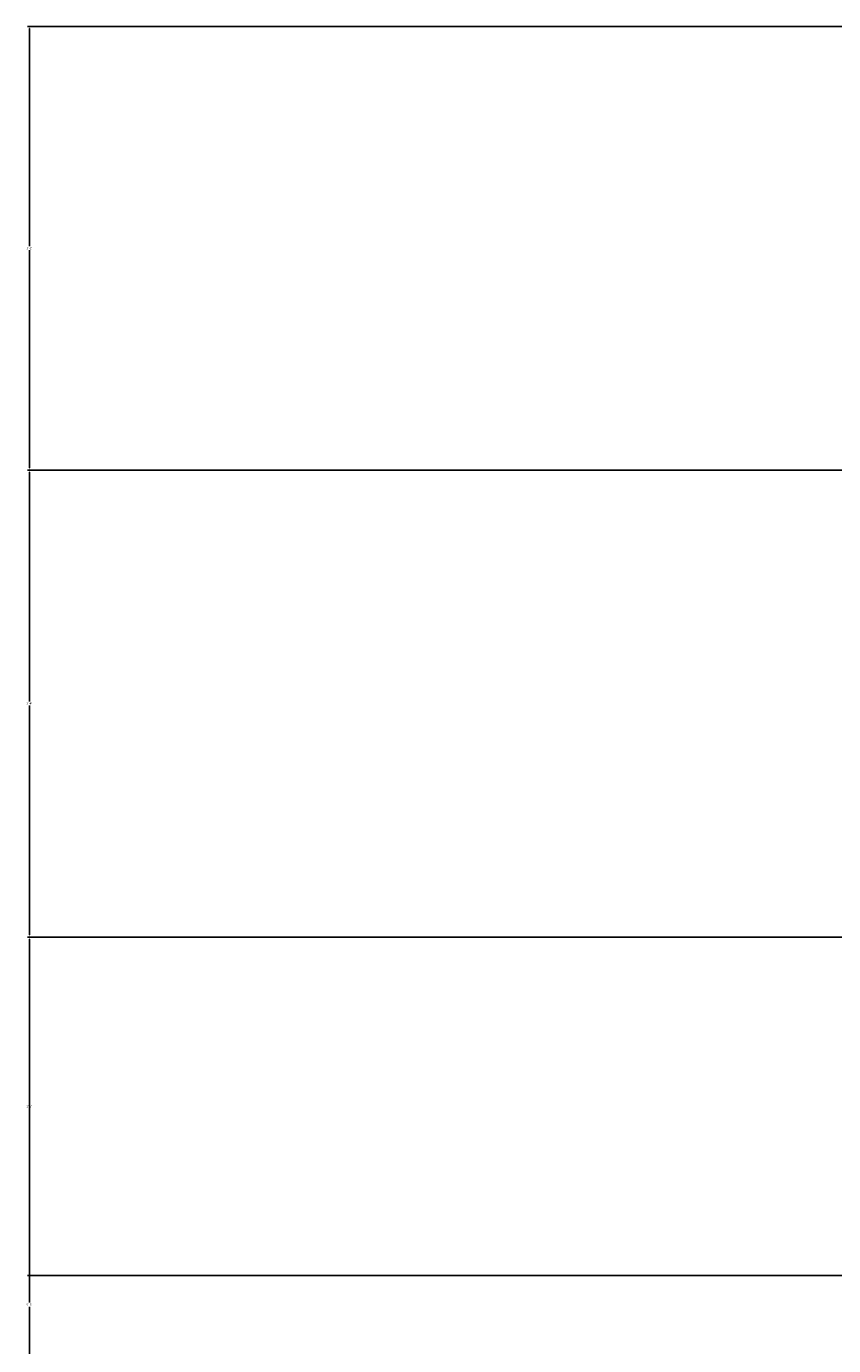
# Model space of a CAD drawing. Units: inches. Extents: x 37 to 824, y -700 to 234.
# Tile 49 of 77: x 78 to 147, y 78 to 191. Entities that reach past the tile are written whole.
import ezdxf

# ---------------------------------------------------------------- set-up
doc = ezdxf.new("R2010")
doc.units = ezdxf.units.IN
doc.header["$MEASUREMENT"] = 0
doc.layers.add('A-ANNO-DIMS', color=2, linetype='Continuous', lineweight=18)
doc.styles.get("Standard").update_dxf_attribs({"font": 'arial.ttf'})
doc.dimstyles.get("Standard").update_dxf_attribs({"dimtxt": 0.18, "dimasz": 0.18, "dimexe": 0.18, "dimexo": 0.0625, "dimgap": 0.09, "dimtad": 0, "dimtih": 1, "dimtoh": 1, "dimdec": 1, "dimzin": 0, "dimdsep": 46, "dimlunit": 4, "dimtxsty": 'Standard', "dimcen": 0.09, "dimadec": 0, "dimazin": 0, "dimtfac": 1, "dimtdec": 1, "dimtofl": 0, "dimtmove": 0, "dimatfit": 3, "dimfxl": 1, "dimtolj": 1, "dimtzin": 0, "dimarcsym": 0})

# ---------------------------------------------------------------- blocks, each defined once
blk = doc.blocks.new('*D49')
at = {"layer": 'A-ANNO-DIMS', "color": 0, "lineweight": -2, "ltscale": 0.5, "transparency": 16777216}
for p, q in [((161.01, 191.09), (78.16, 191.09)), ((78.34, 190.91), (78.34, 172.27)), ((78.34, 153.27), (78.34, 171.91)), ((161.01, 153.09), (78.16, 153.09))]:
    blk.add_line(p, q, dxfattribs=at)
at = {"layer": 'A-ANNO-DIMS', "color": 0, "ltscale": 0.5, "transparency": 16777216}
for points in [[(78.31, 190.91), (78.37, 190.91), (78.34, 191.09)], [(78.31, 153.27), (78.37, 153.27), (78.34, 153.09)]]:
    blk.add_solid(points, dxfattribs=at)
at = {"layer": 'Defpoints', "color": 0, "ltscale": 0.5, "transparency": 16777216}
for p in [(161.08, 191.09), (78.34, 153.09), (161.08, 153.09)]:
    blk.add_point(p, dxfattribs=at)
at = {"layer": 'A-ANNO-DIMS', "color": 0, "ltscale": 0.5, "transparency": 16777216, "insert": (78.34, 172.09), "char_height": 0.18, "attachment_point": 5}
blk.add_mtext('\\A1;3\'-2"', dxfattribs=at)
blk = doc.blocks.new('*D50')
at = {"layer": 'A-ANNO-DIMS', "color": 0, "lineweight": -2, "ltscale": 0.5, "transparency": 16777216}
for p, q in [((161.01, 153.09), (78.16, 153.09)), ((78.34, 152.91), (78.34, 133.27)), ((78.34, 113.27), (78.34, 132.91)), ((161.01, 113.09), (78.16, 113.09))]:
    blk.add_line(p, q, dxfattribs=at)
at = {"layer": 'A-ANNO-DIMS', "color": 0, "ltscale": 0.5, "transparency": 16777216}
for points in [[(78.31, 152.91), (78.37, 152.91), (78.34, 153.09)], [(78.31, 113.27), (78.37, 113.27), (78.34, 113.09)]]:
    blk.add_solid(points, dxfattribs=at)
at = {"layer": 'Defpoints', "color": 0, "ltscale": 0.5, "transparency": 16777216}
for p in [(161.08, 153.09), (78.34, 113.09), (161.08, 113.09)]:
    blk.add_point(p, dxfattribs=at)
at = {"layer": 'A-ANNO-DIMS', "color": 0, "ltscale": 0.5, "transparency": 16777216, "insert": (78.34, 133.09), "char_height": 0.18, "attachment_point": 5}
blk.add_mtext('\\A1;3\'-4"', dxfattribs=at)
blk = doc.blocks.new('*D51')
at = {"layer": 'A-ANNO-DIMS', "color": 0, "lineweight": -2, "ltscale": 0.5, "transparency": 16777216}
for p, q in [((161.01, 113.09), (78.16, 113.09)), ((78.34, 112.91), (78.34, 81.77)), ((78.34, 50.27), (78.34, 81.41)), ((161.01, 50.09), (78.16, 50.09))]:
    blk.add_line(p, q, dxfattribs=at)
at = {"layer": 'A-ANNO-DIMS', "color": 0, "ltscale": 0.5, "transparency": 16777216}
for points in [[(78.31, 112.91), (78.37, 112.91), (78.34, 113.09)], [(78.31, 50.27), (78.37, 50.27), (78.34, 50.09)]]:
    blk.add_solid(points, dxfattribs=at)
at = {"layer": 'Defpoints', "color": 0, "ltscale": 0.5, "transparency": 16777216}
for p in [(161.08, 113.09), (78.34, 50.09), (161.08, 50.09)]:
    blk.add_point(p, dxfattribs=at)
at = {"layer": 'A-ANNO-DIMS', "color": 0, "ltscale": 0.5, "transparency": 16777216, "insert": (78.34, 81.59), "char_height": 0.18, "attachment_point": 5}
blk.add_mtext('\\A1;5\'-3"', dxfattribs=at)
blk = doc.blocks.new('*D60')
at = {"layer": 'A-ANNO-DIMS', "color": 0, "lineweight": -2, "ltscale": 0.5, "transparency": 16777216}
for p, q in [((419.01, 113.09), (78.16, 113.09)), ((78.34, 112.91), (78.34, 98.77)), ((78.34, 84.27), (78.34, 98.41)), ((419.01, 84.09), (78.16, 84.09))]:
    blk.add_line(p, q, dxfattribs=at)
at = {"layer": 'A-ANNO-DIMS', "color": 0, "ltscale": 0.5, "transparency": 16777216}
for points in [[(78.31, 112.91), (78.37, 112.91), (78.34, 113.09)], [(78.31, 84.27), (78.37, 84.27), (78.34, 84.09)]]:
    blk.add_solid(points, dxfattribs=at)
at = {"layer": 'Defpoints', "color": 0, "ltscale": 0.5, "transparency": 16777216}
for p in [(78.34, 113.09), (419.08, 113.09), (419.08, 84.09)]:
    blk.add_point(p, dxfattribs=at)
at = {"layer": 'A-ANNO-DIMS', "color": 0, "ltscale": 0.5, "transparency": 16777216, "insert": (78.34, 98.59), "char_height": 0.18, "attachment_point": 5}
blk.add_mtext('\\A1;2\'-5"', dxfattribs=at)

msp = doc.modelspace()

# ---------------------------------------------------------------- dimensions: what is measured, and where the dimension line sits
at = {"layer": 'A-ANNO-DIMS', "ltscale": 0.5}
for base, p1, p2, picture, middle in [((78.34, 153.09), (161.08, 191.09), (161.08, 153.09), '*D49', (78.34, 172.09)), ((78.34, 113.09), (161.08, 153.09), (161.08, 113.09), '*D50', (78.34, 133.09)), ((78.34, 50.09), (161.08, 113.09), (161.08, 50.09), '*D51', (78.34, 81.59)), ((78.34, 113.09), (419.08, 84.09), (419.08, 113.09), '*D60', (78.34, 98.59))]:
    dim = msp.add_linear_dim(base=base, p1=p1, p2=p2, angle=90, dimstyle='Standard', override={"dimdec": 1, "dimlfac": 1, "dimrnd": 0, "dimzin": 1, "dimdsep": 46, "dimlunit": 4, "dimfrac": 2}, dxfattribs=at)
    dim.commit()
    dim.dimension.update_dxf_attribs({"geometry": picture, "text_midpoint": middle})

doc.saveas('drawing.dxf')
